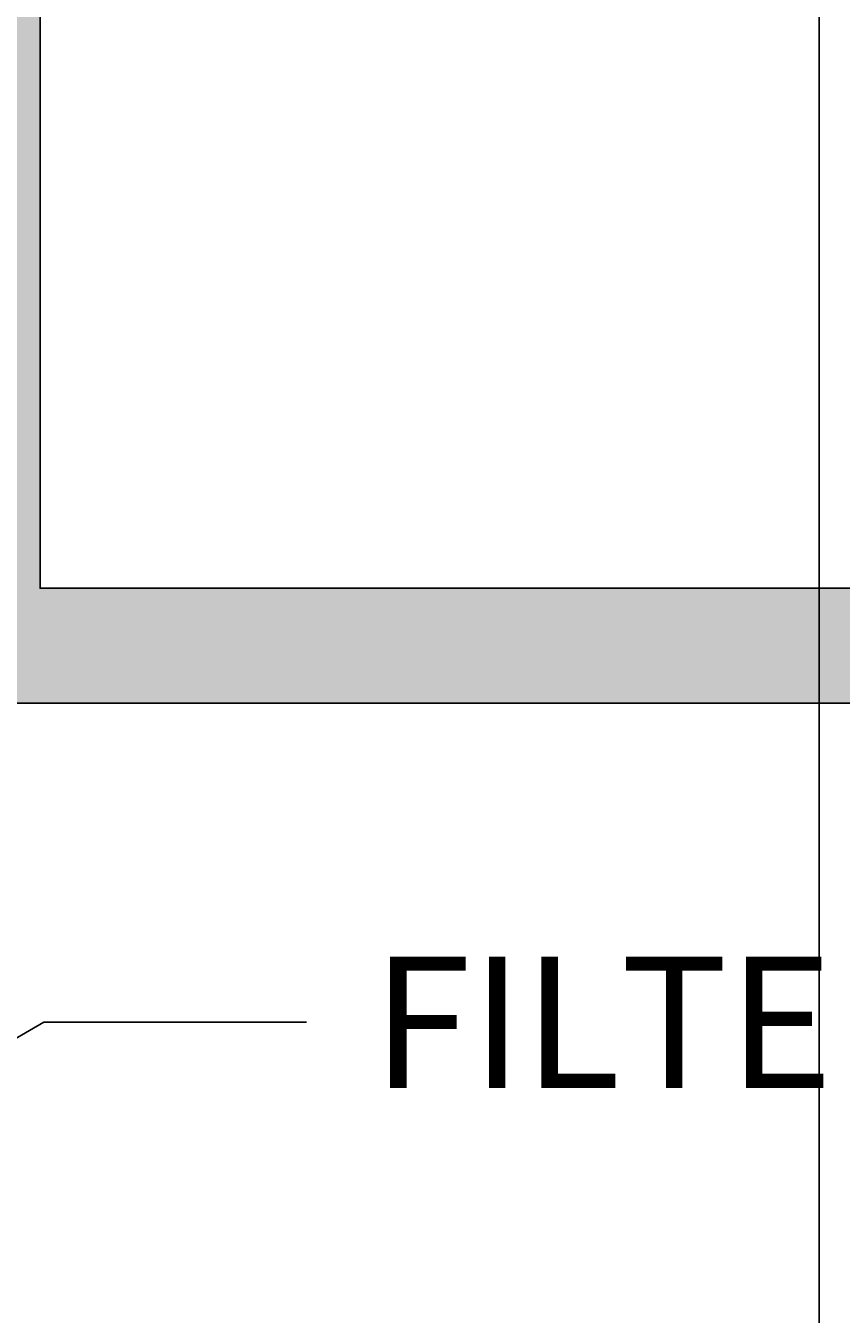
# Model space of a CAD drawing. Units: millimetres. Extents: x -11 to 280, y -4 to 208.
# Tile 9 of 55: x 42 to 67, y 87 to 126. Entities that reach past the tile are written whole.
import ezdxf
from ezdxf import colors
from ezdxf.entities.mleader import LeaderData, LeaderLine
from ezdxf.math import Vec2, Vec3

# ---------------------------------------------------------------- set-up
doc = ezdxf.new("R2010")
doc.units = ezdxf.units.MM
for name, color, linetype, lineweight in [('M-ANNO-TEXT', 7, 'Continuous', 18), ('M-DIMS', 2, 'Continuous', 18), ('M-HYDR-SUCT', 7, 'Continuous', 25)]:
    doc.layers.add(name, color=color, linetype=linetype, lineweight=lineweight)
doc.layers.add('M-HYDR-SUCT-PATT', color=221, linetype='Continuous', lineweight=13, true_color=0xff7fdf)
doc.styles.get("Standard").update_dxf_attribs({"font": 'arial.ttf'})
doc.dimstyles.get("Standard").update_dxf_attribs({"dimtxt": 0.18, "dimasz": 0.18, "dimexe": 0.18, "dimexo": 0.0625, "dimgap": 0.09, "dimtad": 0, "dimtih": 1, "dimtoh": 1, "dimdec": 4, "dimzin": 0, "dimdsep": 46, "dimtxsty": 'Standard', "dimcen": 0.09, "dimadec": 0, "dimazin": 0, "dimtfac": 1, "dimtdec": 4, "dimtofl": 0, "dimtmove": 0, "dimatfit": 3, "dimfxl": 1, "dimtolj": 1, "dimtzin": 0, "dimarcsym": 0})

# ---------------------------------------------------------------- blocks, each defined once
blk = doc.blocks.new('*D5')
at = {"layer": 'Defpoints', "color": 0, "transparency": 16777216}
for p in [(24.759, 192.645), (-10.087, 11.435), (261.686, 11.435)]:
    blk.add_point(p, dxfattribs=at)
at = {"layer": 'M-DIMS', "color": 0, "lineweight": -2, "transparency": 16777216}
for p, q in [((24.696, 192.645), (-10.267, 192.645)), ((-10.087, 192.465), (-10.087, 102.222)), ((-10.087, 11.615), (-10.087, 101.858)), ((261.624, 11.435), (-10.267, 11.435))]:
    blk.add_line(p, q, dxfattribs=at)
at = {"layer": 'M-DIMS', "color": 0, "transparency": 16777216}
for points in [[(-10.117, 192.465), (-10.057, 192.465), (-10.087, 192.645)], [(-10.117, 11.615), (-10.057, 11.615), (-10.087, 11.435)]]:
    blk.add_solid(points, dxfattribs=at)
at = {"layer": 'M-DIMS', "color": 0, "transparency": 16777216, "insert": (-10.087, 102.04), "char_height": 0.18, "attachment_point": 5}
blk.add_mtext('\\A1;181.2', dxfattribs=at)
blk = doc.blocks.new('*D9')
at = {"layer": 'Defpoints', "color": 0, "transparency": 16777216}
for p in [(78.827, 207.495), (31.006, 98.021), (78.827, 98.149)]:
    blk.add_point(p, dxfattribs=at)
at = {"layer": 'M-DIMS', "color": 0, "lineweight": -2, "transparency": 16777216}
for p, q in [((31.006, 98.084), (31.006, 207.675)), ((31.186, 207.495), (54.52, 207.495)), ((78.647, 207.495), (55.313, 207.495)), ((78.827, 98.212), (78.827, 207.675))]:
    blk.add_line(p, q, dxfattribs=at)
at = {"layer": 'M-DIMS', "color": 0, "transparency": 16777216}
for points in [[(31.186, 207.525), (31.186, 207.465), (31.006, 207.495)], [(78.647, 207.525), (78.647, 207.465), (78.827, 207.495)]]:
    blk.add_solid(points, dxfattribs=at)
at = {"layer": 'M-DIMS', "color": 0, "transparency": 16777216, "insert": (54.917, 207.495), "char_height": 0.18, "attachment_point": 5}
blk.add_mtext('\\A1;47.82', dxfattribs=at)
blk = doc.blocks.new('*D23')
at = {"layer": 'Defpoints', "color": 0, "transparency": 16777216}
for p in [(29.201, 153.977), (66.388, 153.977), (66.388, -3.415)]:
    blk.add_point(p, dxfattribs=at)
at = {"layer": 'M-DIMS', "color": 0, "lineweight": -2, "transparency": 16777216}
for p, q in [((29.201, 153.914), (29.201, -3.595)), ((66.388, 153.914), (66.388, -3.595)), ((29.381, -3.415), (47.331, -3.415)), ((66.208, -3.415), (48.258, -3.415))]:
    blk.add_line(p, q, dxfattribs=at)
at = {"layer": 'M-DIMS', "color": 0, "transparency": 16777216}
for points in [[(29.381, -3.385), (29.381, -3.445), (29.201, -3.415)], [(66.208, -3.385), (66.208, -3.445), (66.388, -3.415)]]:
    blk.add_solid(points, dxfattribs=at)
at = {"layer": 'M-DIMS', "color": 0, "transparency": 16777216, "insert": (47.795, -3.415), "char_height": 0.18, "attachment_point": 5}
blk.add_mtext('\\A1;37.186', dxfattribs=at)

msp = doc.modelspace()

# ---------------------------------------------------------------- hatches: boundary and pattern name
at = {"layer": 'M-HYDR-SUCT-PATT'}
h = msp.add_hatch(color=256, dxfattribs=at)
h.set_gradient(color1=(255, 127, 223), color2=(255, 127, 223), tint=1, name='INVCYLINDER')
h.paths.add_polyline_path([(91.3629, 155.4768), (91.3629, 132.4768), (58.3629, 132.4768), (58.3629, 153.9768), (54.8629, 153.9768), (54.8629, 128.9768), (94.8629, 128.9768), (94.8629, 151.9768), (205.5315, 151.9768), (205.5315, 155.4768)])
h.paths.add_polyline_path([(91.3, 114.9452, 1), (78.8273, 114.9452), (78.8273, 108.8141), (42.6453, 108.8141), (42.6453, 153.9768), (39.1453, 153.9768), (39.1453, 105.3141), (78.8273, 105.3141), (78.8273, 98.1491, 1), (91.3, 98.1491), (91.3, 105.3141), (95.5776, 105.3141), (95.5776, 108.8141), (91.3, 108.8141)])
h.paths.add_polyline_path([(228.7, 138.4081), (232.2, 138.4081), (232.2, 144.6609), (228.7, 144.6609)])
h.paths.add_polyline_path([(253.1005, 151.9768, 1), (253.1005, 155.4768), (252.6001, 155.4768), (253.5249, 153.991, -0.1401047), (253.6005, 153.7268, -0.7542249), (252.676, 153.4626), (251.4221, 155.4768), (236.9353, 155.4768), (236.9353, 151.9768)])
h.paths.add_polyline_path([(30.8182, 40.7626), (30.8182, 36.7626), (60.8182, 36.7626), (60.8182, 40.7626)])

# ---------------------------------------------------------------- linework, layer by layer
at = {"layer": 'M-HYDR-SUCT'}
for points in [[(78.8273, 105.3141), (39.1453, 105.3141), (39.1453, 153.9768)], [(78.8273, 108.8141), (42.6453, 108.8141), (42.6453, 153.9768)]]:
    msp.add_lwpolyline(points, dxfattribs=at)

# ---------------------------------------------------------------- dimensions: what is measured, and where the dimension line sits
at = {"layer": 'M-DIMS'}
for base, p1, p2, override, picture, middle in [((78.8273, 207.495), (31.0059, 98.0213), (78.8273, 98.1491), {"dimdec": 2, "dimlfac": 1, "dimrnd": 0, "dimzin": 0, "dimdsep": 46, "dimlunit": 2}, '*D9', (54.9166, 207.495)), ((66.3875, -3.4154), (29.2015, 153.9768), (66.3875, 153.9768), {"dimdec": 3, "dimlfac": 1, "dimrnd": 0, "dimzin": 0, "dimdsep": 46, "dimlunit": 2}, '*D23', (47.7945, -3.4154))]:
    dim = msp.add_linear_dim(base=base, p1=p1, p2=p2, dimstyle='Standard', override=override, dxfattribs=at)
    dim.commit()
    dim.dimension.update_dxf_attribs({"geometry": picture, "text_midpoint": middle})
dim = msp.add_linear_dim(base=(-10.0865, 11.4346), p1=(24.7588, 192.645), p2=(261.6863, 11.4346), angle=90, dimstyle='Standard', override={"dimdec": 1, "dimlfac": 1, "dimrnd": 0, "dimzin": 0, "dimdsep": 46, "dimlunit": 2}, dxfattribs=at)
dim.commit()
dim.dimension.update_dxf_attribs({"geometry": '*D5', "text_midpoint": (-10.0865, 102.0398)})

# ---------------------------------------------------------------- leaders
at = {"layer": 'M-ANNO-TEXT'}
ml = msp.add_multileader_mtext('Standard', dxfattribs=at)
ml.set_content('FILTER', color=256)
ml.set_leader_properties()
ml.build(insert=Vec2(0, 0))
ctx = ml.context
ctx.base_point, ctx.plane_origin = Vec3(50.7635, 95.5863), Vec3(31.0059, 88.798)
notes = []
notes.append((ctx, [(0, (1, 1, 0), (42.7635, 95.5863), (1, 0), 8, [(0, [(31.0059, 88.798)], 0, [])])]))
ctx.mtext.insert, ctx.mtext.flow_direction = Vec3(52.7635, 97.5863), 5
for ctx, leaders in notes:
    for number, flags, end, landing, length, lines in leaders:
        leader = LeaderData()
        leader.index, (leader.has_last_leader_line, leader.has_dogleg_vector, leader.attachment_direction) = number, flags
        leader.last_leader_point, leader.dogleg_vector, leader.dogleg_length = Vec3(end), Vec3(landing), length
        for number, points, colour, breaks in lines:
            line = LeaderLine()
            line.index, line.vertices, line.color, line.breaks = number, Vec3.list(points), colors.encode_raw_color(colour), breaks
            leader.lines.append(line)
        ctx.leaders.append(leader)

doc.saveas('drawing.dxf')
